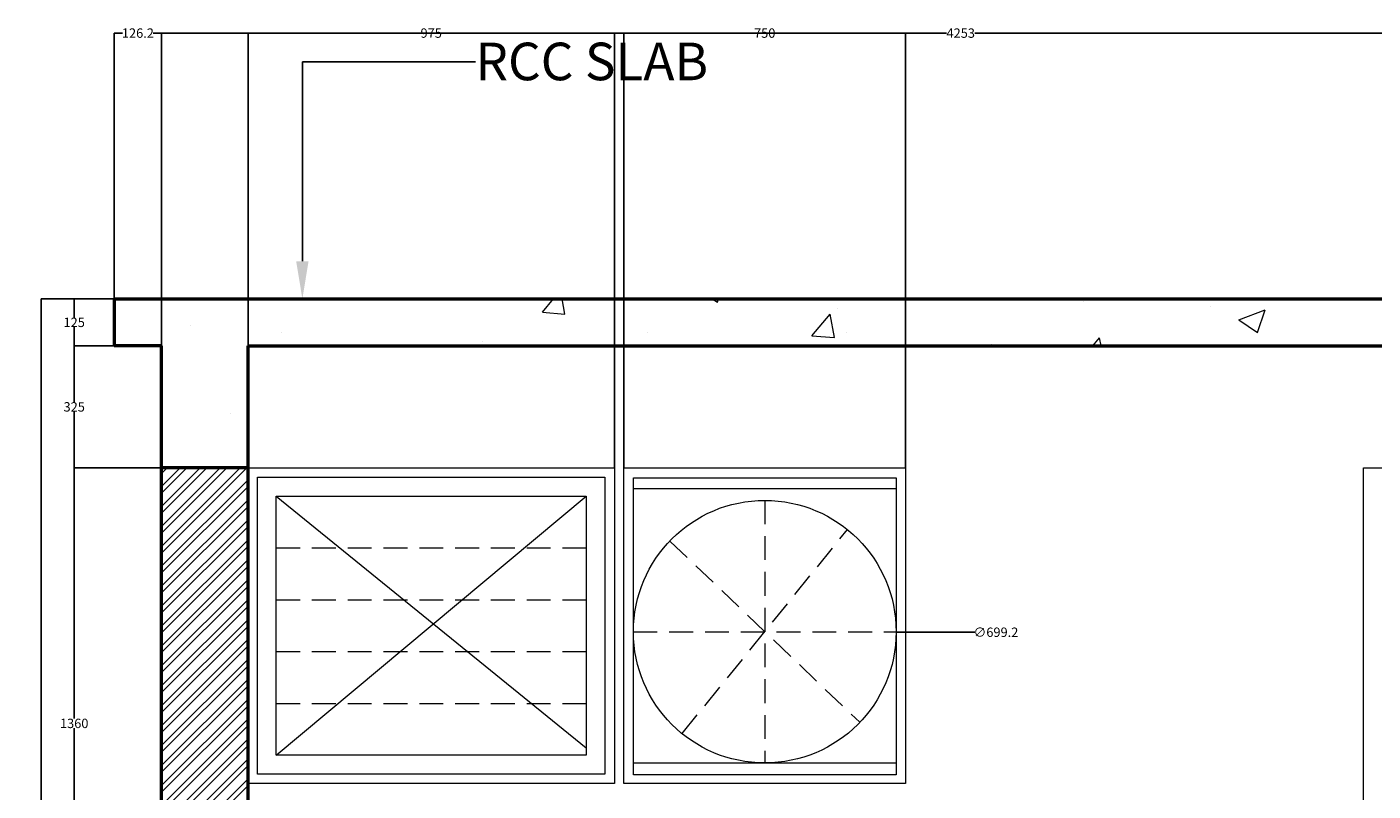
# Model space of a CAD drawing. Units: millimetres. Extents: x 1944 to 29915, y -10550 to 5909.
# Tile 23 of 24: x 19892 to 23475, y 2046 to 4080. Entities that reach past the tile are written whole.
import ezdxf
from ezdxf import colors
from ezdxf.entities.mleader import LeaderData, LeaderLine
from ezdxf.math import Vec2, Vec3

# ---------------------------------------------------------------- set-up
doc = ezdxf.new("R2010")
doc.units = ezdxf.units.MM
doc.header["$MEASUREMENT"] = 0
doc.linetypes.add('HIDDEN', pattern=[9.525, 6.35, -3.175])
for name, color, linetype, lineweight in [('A-ANNO-DIMS', 2, 'Continuous', 18), ('A-ANNO-TEXT', 7, 'Continuous', 25), ('A-ELEV', 3, 'Continuous', 18), ('A-ELEV-HIDN', 3, 'HIDDEN', 13), ('A-WALL', 7, 'Continuous', 50), ('A-WALL-PATT', 8, 'Continuous', 18)]:
    doc.layers.add(name, color=color, linetype=linetype, lineweight=lineweight)
doc.styles.get("Standard").update_dxf_attribs({"font": 'arial.ttf'})
doc.dimstyles.get("Standard").update_dxf_attribs({"dimtxt": 25, "dimasz": 0.18, "dimexe": 0.18, "dimexo": 0.0625, "dimgap": 0.09, "dimtad": 0, "dimtih": 1, "dimtoh": 1, "dimdec": 0, "dimzin": 0, "dimdsep": 46, "dimtxsty": 'Standard', "dimcen": 0.09, "dimadec": 0, "dimazin": 0, "dimtfac": 1, "dimtdec": 0, "dimtofl": 0, "dimtmove": 0, "dimatfit": 3, "dimfxl": 1, "dimtolj": 1, "dimtzin": 0, "dimarcsym": 0})

# ---------------------------------------------------------------- blocks, each defined once
blk = doc.blocks.new('*D18')
at = {"layer": 'A-ANNO-DIMS', "color": 0, "lineweight": -2, "transparency": 16777216}
for p, q in [((20250.8, 2905.8), (20018.1, 2905.8)), ((20018.3, 2905.7), (20018.3, 2238.7)), ((20018.3, 1546), (20018.3, 2213)), ((20250.8, 1545.8), (20018.1, 1545.8))]:
    blk.add_line(p, q, dxfattribs=at)
at = {"layer": 'A-ANNO-DIMS', "color": 0, "transparency": 16777216}
for points in [[(20018.2, 2905.7), (20018.3, 2905.7), (20018.3, 2905.8)], [(20018.2, 1546), (20018.3, 1546), (20018.3, 1545.8)]]:
    blk.add_solid(points, dxfattribs=at)
at = {"layer": 'Defpoints', "color": 0, "transparency": 16777216}
for p in [(20018.3, 2905.8), (20250.9, 2905.8), (20250.9, 1545.8)]:
    blk.add_point(p, dxfattribs=at)
at = {"layer": 'A-ANNO-DIMS', "color": 0, "transparency": 16777216, "insert": (20018.3, 2225.8), "char_height": 25, "attachment_point": 5}
blk.add_mtext('\\A1;1360', dxfattribs=at)
blk = doc.blocks.new('*D19')
at = {"layer": 'A-ANNO-DIMS', "color": 0, "lineweight": -2, "transparency": 16777216}
for p, q in [((20124.6, 3230.8), (20018.1, 3230.8)), ((20018.3, 3230.7), (20018.3, 3081.2)), ((20018.3, 2906), (20018.3, 3055.5)), ((20061.5, 2905.8), (20018.1, 2905.8))]:
    blk.add_line(p, q, dxfattribs=at)
at = {"layer": 'A-ANNO-DIMS', "color": 0, "transparency": 16777216}
for points in [[(20018.3, 3230.7), (20018.3, 3230.7), (20018.3, 3230.8)], [(20018.3, 2906), (20018.3, 2906), (20018.3, 2905.8)]]:
    blk.add_solid(points, dxfattribs=at)
at = {"layer": 'Defpoints', "color": 0, "transparency": 16777216}
for p in [(20018.3, 3230.8), (20124.6, 3230.8), (20061.5, 2905.8)]:
    blk.add_point(p, dxfattribs=at)
at = {"layer": 'A-ANNO-DIMS', "color": 0, "transparency": 16777216, "insert": (20018.3, 3068.3), "char_height": 25, "attachment_point": 5}
blk.add_mtext('\\A1;325', dxfattribs=at)
blk = doc.blocks.new('*D20')
at = {"layer": 'A-ANNO-DIMS', "color": 0, "lineweight": -2, "transparency": 16777216}
for p, q in [((20124.6, 3355.8), (20018.1, 3355.8)), ((20018.3, 3355.7), (20018.3, 3306.2)), ((20018.3, 3231), (20018.3, 3280.5)), ((20124.6, 3230.8), (20018.1, 3230.8))]:
    blk.add_line(p, q, dxfattribs=at)
at = {"layer": 'A-ANNO-DIMS', "color": 0, "transparency": 16777216}
for points in [[(20018.3, 3355.7), (20018.4, 3355.7), (20018.3, 3355.8)], [(20018.3, 3231), (20018.4, 3231), (20018.3, 3230.8)]]:
    blk.add_solid(points, dxfattribs=at)
at = {"layer": 'Defpoints', "color": 0, "transparency": 16777216}
for p in [(20018.3, 3355.8), (20124.6, 3355.8), (20124.6, 3230.8)]:
    blk.add_point(p, dxfattribs=at)
at = {"layer": 'A-ANNO-DIMS', "color": 0, "transparency": 16777216, "insert": (20018.3, 3293.3), "char_height": 25, "attachment_point": 5}
blk.add_mtext('\\A1;125', dxfattribs=at)
blk = doc.blocks.new('*D21')
at = {"layer": 'A-ANNO-DIMS', "color": 0, "lineweight": -2, "transparency": 16777216}
for p, q in [((20124.6, 3355.8), (19930.2, 3355.8)), ((19930.3, 3355.7), (19930.3, 1706.2)), ((19930.3, 31), (19930.3, 1680.5)), ((20061.5, 30.8), (19930.2, 30.8))]:
    blk.add_line(p, q, dxfattribs=at)
at = {"layer": 'A-ANNO-DIMS', "color": 0, "transparency": 16777216}
for points in [[(19930.3, 3355.7), (19930.4, 3355.7), (19930.3, 3355.8)], [(19930.3, 31), (19930.4, 31), (19930.3, 30.8)]]:
    blk.add_solid(points, dxfattribs=at)
at = {"layer": 'Defpoints', "color": 0, "transparency": 16777216}
for p in [(20124.6, 3355.8), (19930.3, 30.8), (20061.5, 30.8)]:
    blk.add_point(p, dxfattribs=at)
at = {"layer": 'A-ANNO-DIMS', "color": 0, "transparency": 16777216, "insert": (19930.3, 1693.3), "char_height": 25, "attachment_point": 5}
blk.add_mtext('\\A1;3325', dxfattribs=at)
blk = doc.blocks.new('*D72')
at = {"layer": 'A-ANNO-DIMS', "color": 0, "lineweight": -2, "transparency": 16777216}
for p, q in [((20124.6, 3230.9), (20124.6, 4063.5)), ((20124.8, 4063.3), (20146.8, 4063.3)), ((20250.7, 4063.3), (20228.7, 4063.3)), ((20250.9, 3230.9), (20250.9, 4063.5))]:
    blk.add_line(p, q, dxfattribs=at)
at = {"layer": 'A-ANNO-DIMS', "color": 0, "transparency": 16777216}
for points in [[(20124.8, 4063.4), (20124.8, 4063.3), (20124.6, 4063.3)], [(20250.7, 4063.4), (20250.7, 4063.3), (20250.9, 4063.3)]]:
    blk.add_solid(points, dxfattribs=at)
at = {"layer": 'Defpoints', "color": 0, "transparency": 16777216}
for p in [(20250.9, 4063.3), (20124.6, 3230.8), (20250.9, 3230.8)]:
    blk.add_point(p, dxfattribs=at)
at = {"layer": 'A-ANNO-DIMS', "color": 0, "transparency": 16777216, "insert": (20187.8, 4063.3), "char_height": 25, "attachment_point": 5}
blk.add_mtext('\\A1;126.2', dxfattribs=at)
blk = doc.blocks.new('*D73')
at = {"layer": 'A-ANNO-DIMS', "color": 0, "lineweight": -2, "transparency": 16777216}
for p, q in [((20250.9, 3230.9), (20250.9, 4063.5)), ((20251, 4063.3), (22339.6, 4063.3)), ((24504, 4063.3), (22415.4, 4063.3)), ((24504.1, 3230.9), (24504.1, 4063.5))]:
    blk.add_line(p, q, dxfattribs=at)
at = {"layer": 'A-ANNO-DIMS', "color": 0, "transparency": 16777216}
for points in [[(20251, 4063.4), (20251, 4063.3), (20250.9, 4063.3)], [(24504, 4063.4), (24504, 4063.3), (24504.1, 4063.3)]]:
    blk.add_solid(points, dxfattribs=at)
at = {"layer": 'Defpoints', "color": 0, "transparency": 16777216}
for p in [(24504.1, 4063.3), (20250.9, 3230.8), (24504.1, 3230.8)]:
    blk.add_point(p, dxfattribs=at)
at = {"layer": 'A-ANNO-DIMS', "color": 0, "transparency": 16777216, "insert": (22377.5, 4063.3), "char_height": 25, "attachment_point": 5}
blk.add_mtext('\\A1;4253', dxfattribs=at)
blk = doc.blocks.new('*D83')
at = {"layer": 'A-ANNO-DIMS', "color": 0, "lineweight": -2, "transparency": 16777216}
for p, q in [((20480.9, 2905.9), (20480.9, 4063.5)), ((20481, 4063.3), (20940.6, 4063.3)), ((21455.7, 4063.3), (20996.2, 4063.3)), ((21455.9, 2905.9), (21455.9, 4063.5))]:
    blk.add_line(p, q, dxfattribs=at)
at = {"layer": 'A-ANNO-DIMS', "color": 0, "transparency": 16777216}
for points in [[(20481, 4063.4), (20481, 4063.3), (20480.9, 4063.3)], [(21455.7, 4063.4), (21455.7, 4063.3), (21455.9, 4063.3)]]:
    blk.add_solid(points, dxfattribs=at)
at = {"layer": 'Defpoints', "color": 0, "transparency": 16777216}
for p in [(21455.9, 4063.3), (20480.9, 2905.8), (21455.9, 2905.8)]:
    blk.add_point(p, dxfattribs=at)
at = {"layer": 'A-ANNO-DIMS', "color": 0, "transparency": 16777216, "insert": (20968.4, 4063.3), "char_height": 25, "attachment_point": 5}
blk.add_mtext('\\A1;975', dxfattribs=at)
blk = doc.blocks.new('*D84')
at = {"layer": 'A-ANNO-DIMS', "color": 0, "lineweight": -2, "transparency": 16777216}
for p, q in [((21480.9, 2905.9), (21480.9, 4063.5)), ((21481, 4063.3), (21828.3, 4063.3)), ((22230.7, 4063.3), (21883.4, 4063.3)), ((22230.9, 2905.9), (22230.9, 4063.5))]:
    blk.add_line(p, q, dxfattribs=at)
at = {"layer": 'A-ANNO-DIMS', "color": 0, "transparency": 16777216}
for points in [[(21481, 4063.4), (21481, 4063.3), (21480.9, 4063.3)], [(22230.7, 4063.4), (22230.7, 4063.3), (22230.9, 4063.3)]]:
    blk.add_solid(points, dxfattribs=at)
at = {"layer": 'Defpoints', "color": 0, "transparency": 16777216}
for p in [(22230.9, 4063.3), (21480.9, 2905.8), (22230.9, 2905.8)]:
    blk.add_point(p, dxfattribs=at)
at = {"layer": 'A-ANNO-DIMS', "color": 0, "transparency": 16777216, "insert": (21855.9, 4063.3), "char_height": 25, "attachment_point": 5}
blk.add_mtext('\\A1;750', dxfattribs=at)
blk = doc.blocks.new('*D100')
at = {"layer": 'A-ANNO-DIMS', "color": 0, "lineweight": -2, "transparency": 16777216}
for p, q in [((21856.1, 2469.9), (21856.3, 2469.9)), ((21856.2, 2469.8), (21856.2, 2470)), ((22415.5, 2468.4), (22205.9, 2469))]:
    blk.add_line(p, q, dxfattribs=at)
at = {"layer": 'A-ANNO-DIMS', "color": 0, "transparency": 16777216}
blk.add_solid([(22205.9, 2469), (22205.9, 2469), (22205.7, 2469)], dxfattribs=at)
at = {"layer": 'Defpoints', "color": 0, "transparency": 16777216}
for p in [(21506.6, 2470.9), (22205.7, 2469)]:
    blk.add_point(p, dxfattribs=at)
at = {"layer": 'A-ANNO-DIMS', "color": 0, "transparency": 16777216, "insert": (22471.2, 2468.4), "char_height": 25, "attachment_point": 5}
blk.add_mtext('\\A1;∅699.2', dxfattribs=at)

msp = doc.modelspace()

# ---------------------------------------------------------------- hatches: boundary and pattern name
at = {"layer": 'A-WALL-PATT'}
h = msp.add_hatch(dxfattribs=at)
h.set_pattern_fill('AR-CONC', color=256, scale=100)
h.paths.add_polyline_path([(24879.698, 3355.837), (20124.649, 3355.837), (20124.649, 3230.837), (20250.858, 3230.837), (20250.858, 2905.837), (20480.858, 2905.837), (20480.858, 3230.837), (24274.139, 3230.837), (24274.139, 2905.837), (24504.139, 2905.837), (24504.139, 3230.837), (24879.698, 3230.837)])
h = msp.add_hatch(dxfattribs=at)
h.set_pattern_fill('ANSI32', color=256, scale=100)
h.paths.add_polyline_path([(20480.858, 2905.837), (20250.858, 2905.837), (20250.858, 30.837), (20480.858, 30.837)])

# ---------------------------------------------------------------- linework, layer by layer
at = {"layer": 'A-ELEV'}
for p, q in [((20555.858, 2830.837), (21380.858, 2161.131)), ((20555.858, 2140.837), (21380.858, 2830.837)), ((21506.584, 2850.837), (22205.436, 2850.837)), ((21506.584, 2120.355), (22205.858, 2120.355))]:
    msp.add_line(p, q, dxfattribs=at)
for points in [[(20480.858, 2905.837), (21455.858, 2905.837), (21455.858, 2065.837), (20480.858, 2065.837)], [(20505.858, 2880.837), (21430.858, 2880.837), (21430.858, 2090.837), (20505.858, 2090.837)], [(21506.584, 2879.763), (22205.436, 2879.774), (22205.436, 2089.292), (21506.584, 2089.28)], [(20555.858, 2830.837), (21380.858, 2830.837), (21380.858, 2140.837), (20555.858, 2140.837)]]:
    msp.add_lwpolyline(points, close=True, dxfattribs=at)
for points in [[(22230.858, 2905.837), (22230.858, 2065.355), (21480.858, 2065.355), (21480.858, 2905.837), (22230.858, 2905.837)], [(23449.139, 30.837), (23449.139, 2905.837), (24249.139, 2905.837)]]:
    msp.add_lwpolyline(points, dxfattribs=at)
msp.add_circle((21856.163, 2469.933), 349.578, dxfattribs=at)
at = {"layer": 'A-ELEV-HIDN', "ltscale": 10}
for p, q in [((21856.163, 2819.511), (21856.163, 2120.355)), ((21636.592, 2198.84), (22076.53, 2742.01)), ((20555.858, 2692.837), (21380.858, 2692.837)), ((21603.637, 2711.025), (22108.688, 2228.841)), ((20555.858, 2554.837), (21380.858, 2554.837)), ((21506.584, 2469.933), (22205.741, 2469.933)), ((20555.858, 2416.837), (21380.858, 2416.837)), ((20555.858, 2278.837), (21380.858, 2278.837))]:
    msp.add_line(p, q, dxfattribs=at)
at = {"layer": 'A-WALL'}
for p, q in [((20124.649, 3355.837), (24879.698, 3355.837)), ((20124.649, 3355.837), (20124.649, 3230.837)), ((20250.858, 3230.837), (20124.649, 3230.837)), ((20250.858, 30.837), (20250.858, 3230.837)), ((20480.858, 30.837), (20480.858, 3230.837)), ((20480.858, 3230.837), (24274.139, 3230.837)), ((20480.858, 2905.837), (20250.858, 2905.837))]:
    msp.add_line(p, q, dxfattribs=at)

# ---------------------------------------------------------------- dimensions: what is measured, and where the dimension line sits
at = {"layer": 'A-ANNO-DIMS'}
for base, p1, p2, override, picture, middle in [((20250.858, 4063.337), (20124.649, 3230.837), (20250.858, 3230.837), {"dimdec": 1, "dimlfac": 1, "dimrnd": 0, "dimzin": 0, "dimdsep": 46, "dimlunit": 2}, '*D72', (20187.753, 4063.337)), ((24504.139, 4063.337), (20250.858, 3230.837), (24504.139, 3230.837), {"dimdec": 0, "dimlfac": 1, "dimrnd": 0, "dimzin": 0, "dimdsep": 46, "dimlunit": 2}, '*D73', (22377.499, 4063.337)), ((21455.858, 4063.337), (20480.858, 2905.837), (21455.858, 2905.837), {"dimdec": 0, "dimlfac": 1, "dimrnd": 0, "dimzin": 0, "dimdsep": 46, "dimlunit": 2}, '*D83', (20968.358, 4063.337)), ((22230.858, 4063.337), (21480.858, 2905.837), (22230.858, 2905.837), {"dimdec": 0, "dimlfac": 1, "dimrnd": 0, "dimzin": 0, "dimdsep": 46, "dimlunit": 2}, '*D84', (21855.858, 4063.337))]:
    dim = msp.add_linear_dim(base=base, p1=p1, p2=p2, dimstyle='Standard', override=override, dxfattribs=at)
    dim.commit()
    dim.dimension.update_dxf_attribs({"geometry": picture, "text_midpoint": middle})
for base, p1, p2, picture, middle in [((19930.341, 30.837), (20124.649, 3355.837), (20061.543, 30.837), '*D21', (19930.341, 1693.337)), ((20018.33, 3355.837), (20124.649, 3230.837), (20124.649, 3355.837), '*D20', (20018.33, 3293.337)), ((20018.3, 3230.837), (20061.543, 2905.837), (20124.649, 3230.837), '*D19', (20018.3, 3068.337)), ((20018.27, 2905.837), (20250.858, 1545.837), (20250.858, 2905.837), '*D18', (20018.27, 2225.837))]:
    dim = msp.add_linear_dim(base=base, p1=p1, p2=p2, angle=90, dimstyle='Standard', override={"dimclrd": 0, "dimclre": 0, "dimclrt": 0}, dxfattribs=at)
    dim.commit()
    dim.dimension.update_dxf_attribs({"geometry": picture, "text_midpoint": middle})
dim = msp.add_diameter_dim_2p(p1=(21506.586, 2470.868), p2=(22205.74, 2468.998), dimstyle='Standard', override={"dimdec": 1, "dimlfac": 1, "dimrnd": 0, "dimzin": 0, "dimdsep": 46, "dimlunit": 2}, dxfattribs=at)
dim.commit()
dim.dimension.update_dxf_attribs({"geometry": '*D100', "text_midpoint": (22415.486, 2468.437), "dimtype": 163})

# ---------------------------------------------------------------- leaders
at = {"layer": 'A-ANNO-TEXT'}
ml = msp.add_multileader_mtext('Standard', dxfattribs=at)
ml.set_content('RCC SLAB ', color=256)
ml.set_leader_properties()
ml.build(insert=Vec2(0, 0))
ml.multileader.update_dxf_attribs({"dogleg_length": 0.36, "arrow_head_size": 100})
ctx = ml.context
ctx.base_point, ctx.char_height, ctx.arrow_head_size, ctx.landing_gap_size, ctx.plane_origin = Vec3(21086.06, 3986.992), 100, 100, 0.09, Vec3(21085.7, 3986.992)
notes = []
notes.append((ctx, [(0, (1, 1, 0), (21085.7, 3986.992), (1, 0), 0.36, [(0, [(20625.51, 3355.837), (20625.51, 3986.992)], 0, [])])]))
ctx.mtext.insert, ctx.mtext.flow_direction = Vec3(21086.15, 4037.845), 5
for ctx, leaders in notes:
    for number, flags, end, landing, length, lines in leaders:
        leader = LeaderData()
        leader.index, (leader.has_last_leader_line, leader.has_dogleg_vector, leader.attachment_direction) = number, flags
        leader.last_leader_point, leader.dogleg_vector, leader.dogleg_length = Vec3(end), Vec3(landing), length
        for number, points, colour, breaks in lines:
            line = LeaderLine()
            line.index, line.vertices, line.color, line.breaks = number, Vec3.list(points), colors.encode_raw_color(colour), breaks
            leader.lines.append(line)
        ctx.leaders.append(leader)

doc.saveas('drawing.dxf')
